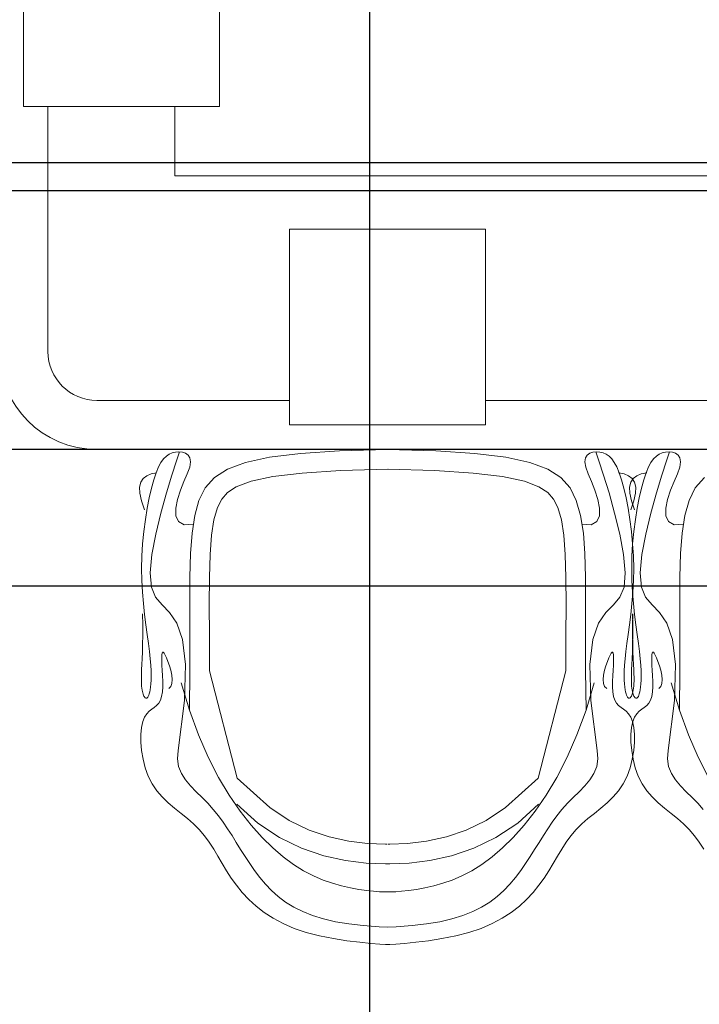
# Model space of a CAD drawing. Units: inches. Extents: x 1454 to 2136, y 626 to 1213.
# Tile 8 of 23: x 1592 to 1620, y 1062 to 1101. Entities that reach past the tile are written whole.
import ezdxf

# ---------------------------------------------------------------- set-up
doc = ezdxf.new("R2010")
doc.units = ezdxf.units.IN
doc.header["$MEASUREMENT"] = 0
for name, color, linetype, lineweight in [('A-ANNO-DIMS', 2, 'Continuous', 18), ('A-FURN-PATT', 252, 'Continuous', 13), ('conference', 41, 'Continuous', 18)]:
    doc.layers.add(name, color=color, linetype=linetype, lineweight=lineweight)
doc.styles.get("Standard").update_dxf_attribs({"font": 'arial.ttf'})
doc.dimstyles.get("Standard").update_dxf_attribs({"dimtxt": 4, "dimasz": 0.18, "dimexe": 0.18, "dimexo": 0.0625, "dimgap": 0.09, "dimtad": 0, "dimtih": 1, "dimtoh": 1, "dimdec": 0, "dimrnd": 6, "dimzin": 0, "dimdsep": 46, "dimlunit": 3, "dimtxsty": 'Standard', "dimcen": 0.09, "dimadec": 0, "dimazin": 0, "dimtfac": 1, "dimtdec": 0, "dimtofl": 0, "dimtmove": 0, "dimatfit": 3, "dimfxl": 1, "dimtolj": 1, "dimtzin": 0, "dimarcsym": 0})

# ---------------------------------------------------------------- blocks, each defined once
blk = doc.blocks.new('ОГ52_на12персон_стол2800х900')
for p, q in [((-1375, -70.7), (-1375, -270.7)), ((-1175, -270.7), (-1175, -70.7)), ((-1375, -270.7), (-1175, -270.7)), ((-1350, -270.7), (-1350, -520.7)), ((-1220.7, -341.4), (-1220.7, -270.7)), ((-1220.7, -341.4), (1220.7, -341.4)), ((-903.4, -395.7), (-1103.4, -395.7)), ((-1103.4, -395.7), (-1103.4, -595.7)), ((-903.4, -595.7), (-903.4, -395.7)), ((-1300, -570.7), (-1103.4, -570.7)), ((-903.4, -570.7), (-603.4, -570.7)), ((-1103.4, -595.7), (-903.4, -595.7)), ((-1300, -620.7), (1300, -620.7)), ((-1216.3, -623.2), (-1219.8, -623.5)), ((-1218.9, -632.3), (-1215.9, -623.2)), ((-1212.8, -623.5), (-1216.3, -623.2)), ((-1092.3, -624.8), (-1052.5, -622.2)), ((-1052.5, -622.2), (-1003.4, -620.7)), ((-954.3, -622.2), (-1003.4, -620.7)), ((-914.4, -624.8), (-954.3, -622.2)), ((-793.9, -623.5), (-790.4, -623.2)), ((-787.8, -632.3), (-790.9, -623.2)), ((-790.4, -623.2), (-786.9, -623.5)), ((-716.3, -623.2), (-719.8, -623.5)), ((-718.9, -632.3), (-715.9, -623.2)), ((-712.8, -623.5), (-716.3, -623.2)), ((-1232, -630.2), (-1234.7, -633.9)), ((-1229.2, -627.4), (-1232, -630.2)), ((-1226.3, -625.5), (-1229.2, -627.4)), ((-1223.2, -624.2), (-1226.3, -625.5)), ((-1223.6, -646.8), (-1218.9, -632.3)), ((-1219.8, -623.5), (-1223.2, -624.2)), ((-1209.6, -624.6), (-1212.8, -623.5)), ((-1207, -626.5), (-1209.6, -624.6)), ((-1205.3, -629.4), (-1207, -626.5)), ((-1204.6, -633.5), (-1205.3, -629.4)), ((-1148.5, -633.9), (-1124, -628.7)), ((-1124, -628.7), (-1092.3, -624.8)), ((-882.8, -628.7), (-914.4, -624.8)), ((-858.3, -633.9), (-882.8, -628.7)), ((-802.1, -633.5), (-801.5, -629.4)), ((-801.5, -629.4), (-799.7, -626.5)), ((-799.7, -626.5), (-797.1, -624.6)), ((-797.1, -624.6), (-793.9, -623.5)), ((-783.1, -646.8), (-787.8, -632.3)), ((-786.9, -623.5), (-783.6, -624.2)), ((-783.6, -624.2), (-780.4, -625.5)), ((-780.4, -625.5), (-777.5, -627.4)), ((-777.5, -627.4), (-774.7, -630.2)), ((-774.7, -630.2), (-772.1, -633.9)), ((-732, -630.2), (-734.7, -633.9)), ((-729.2, -627.4), (-732, -630.2)), ((-726.3, -625.5), (-729.2, -627.4)), ((-723.2, -624.2), (-726.3, -625.5)), ((-723.6, -646.8), (-718.9, -632.3)), ((-719.8, -623.5), (-723.2, -624.2)), ((-709.6, -624.6), (-712.8, -623.5)), ((-707, -626.5), (-709.6, -624.6)), ((-705.3, -629.4), (-707, -626.5)), ((-704.6, -633.5), (-705.3, -629.4)), ((-1237.2, -638.6), (-1239.7, -644.5)), ((-1234.7, -633.9), (-1237.2, -638.6)), ((-1207.8, -645.6), (-1205.4, -638.8)), ((-1205.4, -638.8), (-1204.6, -633.5)), ((-1180.2, -649.4), (-1166.8, -640.7)), ((-1166.8, -640.7), (-1148.5, -633.9)), ((-1090.5, -644.8), (-1051.5, -642.2)), ((-1051.5, -642.2), (-1002.7, -640.7)), ((-955.2, -642.2), (-1004, -640.7)), ((-916.3, -644.8), (-955.2, -642.2)), ((-839.9, -640.7), (-858.3, -633.9)), ((-826.6, -649.4), (-839.9, -640.7)), ((-801.3, -638.8), (-802.1, -633.5)), ((-798.9, -645.6), (-801.3, -638.8)), ((-772.1, -633.9), (-769.5, -638.6)), ((-769.5, -638.6), (-767.1, -644.5)), ((-737.2, -638.6), (-739.7, -644.5)), ((-734.7, -633.9), (-737.2, -638.6)), ((-707.8, -645.6), (-705.4, -638.8)), ((-705.4, -638.8), (-704.6, -633.5)), ((-1255.3, -654.2), (-1252.8, -650.4)), ((-1252.8, -650.4), (-1249.2, -647.6)), ((-1249.2, -647.6), (-1244.6, -645.6)), ((-1244.6, -645.6), (-1239.1, -644.5)), ((-1242.1, -651.7), (-1244.4, -660.3)), ((-1239.7, -644.5), (-1242.1, -651.7)), ((-1229.2, -665.1), (-1223.6, -646.8)), ((-1211.2, -653.4), (-1214.7, -662.3)), ((-1207.8, -645.6), (-1211.2, -653.4)), ((-1189.5, -660), (-1180.2, -649.4)), ((-1157.8, -658.7), (-1142.8, -653.1)), ((-1142.8, -653.1), (-1120.7, -648.4)), ((-1120.7, -648.4), (-1090.5, -644.8)), ((-886.1, -648.4), (-916.3, -644.8)), ((-863.9, -653.1), (-886.1, -648.4)), ((-849, -658.7), (-863.9, -653.1)), ((-817.3, -660), (-826.6, -649.4)), ((-798.9, -645.6), (-795.5, -653.4)), ((-795.5, -653.4), (-792, -662.3)), ((-777.5, -665.1), (-783.1, -646.8)), ((-762.2, -645.6), (-767.7, -644.5)), ((-767.1, -644.5), (-764.7, -651.7)), ((-764.7, -651.7), (-762.3, -660.3)), ((-757.6, -647.6), (-762.2, -645.6)), ((-754, -650.4), (-757.6, -647.6)), ((-755.3, -654.2), (-752.8, -650.4)), ((-751.5, -654.2), (-754, -650.4)), ((-752.8, -650.4), (-749.2, -647.6)), ((-749.2, -647.6), (-744.6, -645.6)), ((-744.6, -645.6), (-739.1, -644.5)), ((-742.1, -651.7), (-744.4, -660.3)), ((-739.7, -644.5), (-742.1, -651.7)), ((-729.2, -665.1), (-723.6, -646.8)), ((-711.2, -653.4), (-714.7, -662.3)), ((-707.8, -645.6), (-711.2, -653.4)), ((-689.5, -660), (-680.2, -649.4)), ((-1256.5, -659.2), (-1255.3, -654.2)), ((-1256.3, -665.5), (-1256.5, -659.2)), ((-1244.4, -660.3), (-1246.6, -670)), ((-1214.7, -662.3), (-1217.7, -671.7)), ((-1195.9, -672.9), (-1189.5, -660)), ((-1166.9, -664.7), (-1157.8, -658.7)), ((-839.8, -664.7), (-849, -658.7)), ((-810.9, -672.9), (-817.3, -660)), ((-792, -662.3), (-789.1, -671.7)), ((-762.3, -660.3), (-760.1, -670)), ((-756.5, -659.2), (-755.3, -654.2)), ((-756.3, -665.5), (-756.5, -659.2)), ((-750.2, -659.2), (-751.5, -654.2)), ((-750.4, -665.5), (-750.2, -659.2)), ((-744.4, -660.3), (-746.6, -670)), ((-714.7, -662.3), (-717.7, -671.7)), ((-695.9, -672.9), (-689.5, -660)), ((-1254.7, -673.2), (-1256.3, -665.5)), ((-1251.4, -682.4), (-1254.7, -673.2)), ((-1246.6, -670), (-1248.7, -680.8)), ((-1235, -685.8), (-1229.2, -665.1)), ((-1217.7, -671.7), (-1219.5, -680.7)), ((-1200.2, -688.1), (-1195.9, -672.9)), ((-1177.1, -680.1), (-1172.7, -671.3)), ((-1172.7, -671.3), (-1166.9, -664.7)), ((-834, -671.3), (-839.8, -664.7)), ((-829.6, -680.1), (-834, -671.3)), ((-806.5, -688.1), (-810.9, -672.9)), ((-789.1, -671.7), (-787.3, -680.7)), ((-771.8, -685.8), (-777.5, -665.1)), ((-760.1, -670), (-758, -680.8)), ((-754.7, -673.2), (-756.3, -665.5)), ((-755.4, -682.4), (-752.1, -673.2)), ((-751.4, -682.4), (-754.7, -673.2)), ((-752.1, -673.2), (-750.4, -665.5)), ((-746.6, -670), (-748.7, -680.8)), ((-735, -685.8), (-729.2, -665.1)), ((-717.7, -671.7), (-719.5, -680.7)), ((-700.2, -688.1), (-695.9, -672.9)), ((-1248.7, -680.8), (-1250.6, -692.3)), ((-1219.5, -680.7), (-1219.4, -688.5)), ((-1180.6, -692.4), (-1177.1, -680.1)), ((-826.1, -692.4), (-829.6, -680.1)), ((-787.3, -680.7), (-787.3, -688.5)), ((-758, -680.8), (-756.2, -692.3)), ((-748.7, -680.8), (-750.6, -692.3)), ((-719.5, -680.7), (-719.4, -688.5)), ((-1250.6, -692.3), (-1252.1, -704.4)), ((-1240.1, -707.3), (-1235, -685.8)), ((-1219.4, -688.5), (-1216.8, -694.3)), ((-1203, -706), (-1200.2, -688.1)), ((-1183.1, -708.3), (-1180.6, -692.4)), ((-823.6, -708.3), (-826.1, -692.4)), ((-803.7, -706), (-806.5, -688.1)), ((-787.3, -688.5), (-789.9, -694.3)), ((-766.6, -707.3), (-771.8, -685.8)), ((-756.2, -692.3), (-754.6, -704.4)), ((-750.6, -692.3), (-752.1, -704.4)), ((-740.1, -707.3), (-735, -685.8)), ((-719.4, -688.5), (-716.8, -694.3)), ((-703, -706), (-700.2, -688.1)), ((-1216.8, -694.3), (-1211.1, -697.5)), ((-1211.1, -697.5), (-1201.6, -697.1)), ((-795.6, -697.5), (-805.1, -697.1)), ((-789.9, -694.3), (-795.6, -697.5)), ((-716.8, -694.3), (-711.1, -697.5)), ((-711.1, -697.5), (-701.6, -697.1)), ((-1252.1, -704.4), (-1253.4, -716.9)), ((-1243.9, -728.1), (-1240.1, -707.3)), ((-1204.6, -726.9), (-1203, -706)), ((-1184.6, -728), (-1183.1, -708.3)), ((-822.1, -728), (-823.6, -708.3)), ((-802.2, -726.9), (-803.7, -706)), ((-762.8, -728.1), (-766.6, -707.3)), ((-754.6, -704.4), (-753.4, -716.9)), ((-752.1, -704.4), (-753.4, -716.9)), ((-743.9, -728.1), (-740.1, -707.3)), ((-704.6, -726.9), (-703, -706)), ((-1253.4, -716.9), (-1254.1, -729.5)), ((-753.4, -716.9), (-754.1, -729.5)), ((-753.4, -716.9), (-752.6, -729.5)), ((-1254.1, -729.5), (-1254.4, -742.1)), ((-1245.6, -746.6), (-1243.9, -728.1)), ((-1205.3, -751.1), (-1204.6, -726.9)), ((-1185.3, -751.4), (-1184.6, -728)), ((-821.5, -751.4), (-822.1, -728)), ((-801.5, -751.1), (-802.2, -726.9)), ((-761.1, -746.6), (-762.8, -728.1)), ((-754.1, -729.5), (-754.4, -742.1)), ((-752.6, -729.5), (-752.3, -742.1)), ((-745.6, -746.6), (-743.9, -728.1)), ((-705.3, -751.1), (-704.6, -726.9)), ((-1254.4, -742.1), (-1254.2, -754.5)), ((-754.4, -742.1), (-754.2, -754.5)), ((-752.3, -742.1), (-752.5, -754.5)), ((-1244.5, -761.4), (-1245.6, -746.6)), ((-1205.4, -778.9), (-1205.3, -751.1)), ((-1185.4, -778.9), (-1185.3, -751.4)), ((-821.4, -778.9), (-821.5, -751.4)), ((-801.4, -778.9), (-801.5, -751.1)), ((-762.2, -761.4), (-761.1, -746.6)), ((-744.5, -761.4), (-745.6, -746.6)), ((-705.4, -778.9), (-705.3, -751.1)), ((-1254.2, -754.5), (-1253.6, -766.5)), ((-1240.2, -771.5), (-1244.5, -761.4)), ((-766.5, -771.5), (-762.2, -761.4)), ((-754.2, -754.5), (-753.6, -766.5)), ((-752.5, -754.5), (-753.1, -766.5)), ((-740.2, -771.5), (-744.5, -761.4)), ((-1253.6, -766.5), (-1252.6, -778.1)), ((-1233.6, -779.2), (-1240.2, -771.5)), ((-773.1, -779.2), (-766.5, -771.5)), ((-753.1, -766.5), (-754.1, -778.1)), ((-753.6, -766.5), (-752.6, -778.1)), ((-733.6, -779.2), (-740.2, -771.5)), ((-1252.6, -778.1), (-1251.4, -789.2)), ((-1226, -787), (-1233.6, -779.2)), ((-1205.3, -810.6), (-1205.4, -778.9)), ((-1185.3, -810.5), (-1185.4, -778.9)), ((-821.5, -810.5), (-821.4, -778.9)), ((-801.5, -810.6), (-801.4, -778.9)), ((-780.7, -787), (-773.1, -779.2)), ((-754.1, -778.1), (-755.4, -789.2)), ((-752.6, -778.1), (-751.4, -789.2)), ((-726, -787), (-733.6, -779.2)), ((-705.3, -810.6), (-705.4, -778.9)), ((-1253.3, -800.2), (-1253.4, -788.5)), ((-1251.4, -789.2), (-1250, -799.7)), ((-1218.6, -798), (-1226, -787)), ((-788.1, -798), (-780.7, -787)), ((-755.4, -789.2), (-756.7, -799.7)), ((-753.5, -800.2), (-753.3, -788.5)), ((-753.3, -800.2), (-753.4, -788.5)), ((-751.4, -789.2), (-750, -799.7)), ((-718.6, -798), (-726, -787)), ((-1253.3, -810.5), (-1253.3, -800.2)), ((-1250, -799.7), (-1248.7, -809.6)), ((-1212.8, -814.7), (-1218.6, -798)), ((-794, -814.7), (-788.1, -798)), ((-756.7, -799.7), (-758, -809.6)), ((-753.4, -810.5), (-753.5, -800.2)), ((-753.3, -810.5), (-753.3, -800.2)), ((-750, -799.7), (-748.7, -809.6)), ((-712.8, -814.7), (-718.6, -798)), ((-1253.4, -819.6), (-1253.3, -810.5)), ((-1248.7, -809.6), (-1247.4, -818.7)), ((-1205.3, -846.4), (-1205.3, -810.6)), ((-1185.3, -846.6), (-1185.3, -810.5)), ((-821.5, -846.6), (-821.5, -810.5)), ((-801.5, -846.4), (-801.5, -810.6)), ((-758, -809.6), (-759.3, -818.7)), ((-753.3, -819.6), (-753.4, -810.5)), ((-753.4, -819.6), (-753.3, -810.5)), ((-748.7, -809.6), (-747.4, -818.7)), ((-705.3, -846.4), (-705.3, -810.6)), ((-1253.7, -827.5), (-1253.4, -819.6)), ((-1247.4, -818.7), (-1246.4, -827)), ((-1209.7, -840.1), (-1212.8, -814.7)), ((-797, -840.1), (-794, -814.7)), ((-759.3, -818.7), (-760.4, -827)), ((-753.7, -827.5), (-753.4, -819.6)), ((-753.1, -827.5), (-753.3, -819.6)), ((-747.4, -818.7), (-746.4, -827)), ((-709.7, -840.1), (-712.8, -814.7)), ((-1254.2, -840.3), (-1253.9, -834.3)), ((-1253.9, -834.3), (-1253.7, -827.5)), ((-1246.4, -827), (-1245.6, -834.4)), ((-1233.8, -830.5), (-1233.9, -833.2)), ((-1233.9, -833.2), (-1233.9, -836.7)), ((-1233.5, -828.6), (-1233.8, -830.5)), ((-1233, -827.7), (-1233.5, -828.6)), ((-1232.3, -827.8), (-1233, -827.7)), ((-1231.4, -828.7), (-1232.3, -827.8)), ((-1230.3, -830.6), (-1231.4, -828.7)), ((-1229, -833.4), (-1230.3, -830.6)), ((-1227.6, -837.1), (-1229, -833.4)), ((-779.2, -837.1), (-777.7, -833.4)), ((-777.7, -833.4), (-776.4, -830.6)), ((-776.4, -830.6), (-775.3, -828.7)), ((-775.3, -828.7), (-774.4, -827.8)), ((-774.4, -827.8), (-773.8, -827.7)), ((-773.8, -827.7), (-773.3, -828.6)), ((-773.3, -828.6), (-772.9, -830.5)), ((-772.9, -830.5), (-772.8, -833.2)), ((-772.8, -833.2), (-772.9, -836.7)), ((-760.4, -827), (-761.2, -834.4)), ((-754.2, -840.3), (-753.9, -834.3)), ((-753.9, -834.3), (-753.7, -827.5)), ((-752.8, -834.3), (-753.1, -827.5)), ((-752.5, -840.3), (-752.8, -834.3)), ((-746.4, -827), (-745.6, -834.4)), ((-733.8, -830.5), (-733.9, -833.2)), ((-733.9, -833.2), (-733.9, -836.7)), ((-733.5, -828.6), (-733.8, -830.5)), ((-733, -827.7), (-733.5, -828.6)), ((-732.3, -827.8), (-733, -827.7)), ((-731.4, -828.7), (-732.3, -827.8)), ((-730.3, -830.6), (-731.4, -828.7)), ((-729, -833.4), (-730.3, -830.6)), ((-727.6, -837.1), (-729, -833.4)), ((-1254.5, -845.4), (-1254.2, -840.3)), ((-1245.6, -834.4), (-1245.1, -841)), ((-1245.1, -841), (-1244.8, -846.8)), ((-1233.9, -836.7), (-1233.7, -841.2)), ((-1233.7, -841.2), (-1233.4, -846.2)), ((-1226.1, -841.5), (-1227.6, -837.1)), ((-1224.7, -846.2), (-1226.1, -841.5)), ((-1210.8, -876.9), (-1209.7, -840.1)), ((-796, -876.9), (-797, -840.1)), ((-782, -846.2), (-780.7, -841.5)), ((-780.7, -841.5), (-779.2, -837.1)), ((-773.1, -841.2), (-773.4, -846.2)), ((-772.9, -836.7), (-773.1, -841.2)), ((-761.7, -841), (-762, -846.8)), ((-761.2, -834.4), (-761.7, -841)), ((-754.5, -845.4), (-754.2, -840.3)), ((-752.3, -845.4), (-752.5, -840.3)), ((-745.6, -834.4), (-745.1, -841)), ((-745.1, -841), (-744.8, -846.8)), ((-733.9, -836.7), (-733.7, -841.2)), ((-733.7, -841.2), (-733.4, -846.2)), ((-726.1, -841.5), (-727.6, -837.1)), ((-724.7, -846.2), (-726.1, -841.5)), ((-710.8, -876.9), (-709.7, -840.1)), ((-1254.7, -853.7), (-1254.6, -849.8)), ((-1254.7, -857), (-1254.7, -853.7)), ((-1254.6, -849.8), (-1254.5, -845.4)), ((-1244.8, -846.8), (-1244.7, -851.9)), ((-1244.7, -851.9), (-1244.8, -856.3)), ((-1233.4, -846.2), (-1233.1, -851.7)), ((-1233.1, -851.7), (-1232.9, -857.3)), ((-1223.7, -851), (-1224.7, -846.2)), ((-1223.3, -855.5), (-1223.7, -851)), ((-1205.7, -886.8), (-1205.3, -846.4)), ((-1157, -956.4), (-1185.3, -846.6)), ((-849.8, -956.4), (-821.5, -846.6)), ((-801, -886.8), (-801.5, -846.4)), ((-783.5, -855.5), (-783, -851)), ((-783, -851), (-782, -846.2)), ((-773.6, -851.7), (-773.8, -857.3)), ((-773.4, -846.2), (-773.6, -851.7)), ((-762, -846.8), (-762, -851.9)), ((-762, -851.9), (-761.9, -856.3)), ((-754.7, -853.7), (-754.6, -849.8)), ((-754.7, -857), (-754.7, -853.7)), ((-754.6, -849.8), (-754.5, -845.4)), ((-752.1, -849.8), (-752.3, -845.4)), ((-752, -853.7), (-752.1, -849.8)), ((-752, -857), (-752, -853.7)), ((-744.8, -846.8), (-744.7, -851.9)), ((-744.7, -851.9), (-744.8, -856.3)), ((-733.4, -846.2), (-733.1, -851.7)), ((-733.1, -851.7), (-732.9, -857.3)), ((-723.7, -851), (-724.7, -846.2)), ((-723.3, -855.5), (-723.7, -851)), ((-705.7, -886.8), (-705.3, -846.4)), ((-1254.6, -859.9), (-1254.7, -857)), ((-1254.5, -862.4), (-1254.6, -859.9)), ((-1254.2, -864.5), (-1254.5, -862.4)), ((-1254, -866.3), (-1254.2, -864.5)), ((-1245.3, -863.3), (-1245.7, -866)), ((-1245, -860.1), (-1245.3, -863.3)), ((-1244.8, -856.3), (-1245, -860.1)), ((-1232.9, -862.9), (-1233.3, -868.2)), ((-1232.9, -857.3), (-1232.9, -862.9)), ((-1226.8, -864.8), (-1224.6, -862.7)), ((-1224.6, -862.7), (-1223.5, -859.6)), ((-1223.5, -859.6), (-1223.3, -855.5)), ((-1214, -859), (-1205.7, -886.8)), ((-792.7, -859), (-801, -886.8)), ((-783.2, -859.6), (-783.5, -855.5)), ((-782.1, -862.7), (-783.2, -859.6)), ((-779.9, -864.8), (-782.1, -862.7)), ((-773.8, -857.3), (-773.8, -862.9)), ((-773.8, -862.9), (-773.5, -868.2)), ((-761.9, -856.3), (-761.7, -860.1)), ((-761.7, -860.1), (-761.4, -863.3)), ((-761.4, -863.3), (-761, -866)), ((-754.6, -859.9), (-754.7, -857)), ((-754.5, -862.4), (-754.6, -859.9)), ((-754.2, -864.5), (-754.5, -862.4)), ((-754, -866.3), (-754.2, -864.5)), ((-752.8, -866.3), (-752.5, -864.5)), ((-752.5, -864.5), (-752.3, -862.4)), ((-752.3, -862.4), (-752.1, -859.9)), ((-752.1, -859.9), (-752, -857)), ((-745.3, -863.3), (-745.7, -866)), ((-745, -860.1), (-745.3, -863.3)), ((-744.8, -856.3), (-745, -860.1)), ((-732.9, -862.9), (-733.3, -868.2)), ((-732.9, -857.3), (-732.9, -862.9)), ((-726.8, -864.8), (-724.6, -862.7)), ((-724.6, -862.7), (-723.5, -859.6)), ((-723.5, -859.6), (-723.3, -855.5)), ((-714, -859), (-705.7, -886.8)), ((-1253.6, -867.9), (-1254, -866.3)), ((-1253.3, -869.2), (-1253.6, -867.9)), ((-1252.9, -870.5), (-1253.3, -869.2)), ((-1252.5, -871.6), (-1252.9, -870.5)), ((-1252.1, -872.5), (-1252.5, -871.6)), ((-1251.6, -873.3), (-1252.1, -872.5)), ((-1251.2, -873.9), (-1251.6, -873.3)), ((-1250.7, -874.3), (-1251.2, -873.9)), ((-1250.2, -874.6), (-1250.7, -874.3)), ((-1248.7, -874.3), (-1249.2, -874.6)), ((-1248.1, -873.7), (-1248.7, -874.3)), ((-1247.6, -872.9), (-1248.1, -873.7)), ((-1247.1, -871.7), (-1247.6, -872.9)), ((-1246.6, -870.2), (-1247.1, -871.7)), ((-1246.2, -868.3), (-1246.6, -870.2)), ((-1245.7, -866), (-1246.2, -868.3)), ((-1234, -872.9), (-1235.2, -876.8)), ((-1233.3, -868.2), (-1234, -872.9)), ((-773.5, -868.2), (-772.8, -872.9)), ((-772.8, -872.9), (-771.6, -876.8)), ((-761, -866), (-760.6, -868.3)), ((-760.6, -868.3), (-760.1, -870.2)), ((-760.1, -870.2), (-759.6, -871.7)), ((-759.6, -871.7), (-759.1, -872.9)), ((-759.1, -872.9), (-758.6, -873.7)), ((-758.6, -873.7), (-758.1, -874.3)), ((-758.1, -874.3), (-757.6, -874.6)), ((-756.5, -874.6), (-756, -874.3)), ((-756, -874.3), (-755.6, -873.9)), ((-755.6, -873.9), (-755.1, -873.3)), ((-755.1, -873.3), (-754.7, -872.5)), ((-754.7, -872.5), (-754.2, -871.6)), ((-754.2, -871.6), (-753.8, -870.5)), ((-753.6, -867.9), (-754, -866.3)), ((-753.8, -870.5), (-753.5, -869.2)), ((-753.3, -869.2), (-753.6, -867.9)), ((-753.5, -869.2), (-753.1, -867.9)), ((-752.9, -870.5), (-753.3, -869.2)), ((-753.1, -867.9), (-752.8, -866.3)), ((-752.5, -871.6), (-752.9, -870.5)), ((-752.1, -872.5), (-752.5, -871.6)), ((-751.6, -873.3), (-752.1, -872.5)), ((-751.2, -873.9), (-751.6, -873.3)), ((-750.7, -874.3), (-751.2, -873.9)), ((-750.2, -874.6), (-750.7, -874.3)), ((-748.7, -874.3), (-749.2, -874.6)), ((-748.1, -873.7), (-748.7, -874.3)), ((-747.6, -872.9), (-748.1, -873.7)), ((-747.1, -871.7), (-747.6, -872.9)), ((-746.6, -870.2), (-747.1, -871.7)), ((-746.2, -868.3), (-746.6, -870.2)), ((-745.7, -866), (-746.2, -868.3)), ((-734, -872.9), (-735.2, -876.8)), ((-733.3, -868.2), (-734, -872.9)), ((-1249.7, -874.7), (-1250.2, -874.6)), ((-1249.2, -874.6), (-1249.7, -874.7)), ((-1241.5, -884.1), (-1244.1, -886)), ((-1239.1, -882.2), (-1241.5, -884.1)), ((-1236.9, -879.9), (-1239.1, -882.2)), ((-1235.2, -876.8), (-1236.9, -879.9)), ((-1217.1, -927.9), (-1210.8, -876.9)), ((-789.6, -927.9), (-796, -876.9)), ((-771.6, -876.8), (-769.8, -879.9)), ((-769.8, -879.9), (-767.7, -882.2)), ((-767.7, -882.2), (-765.2, -884.1)), ((-765.2, -884.1), (-762.6, -886)), ((-757.6, -874.6), (-757, -874.7)), ((-757, -874.7), (-756.5, -874.6)), ((-749.7, -874.7), (-750.2, -874.6)), ((-749.2, -874.6), (-749.7, -874.7)), ((-741.5, -884.1), (-744.1, -886)), ((-739.1, -882.2), (-741.5, -884.1)), ((-736.9, -879.9), (-739.1, -882.2)), ((-735.2, -876.8), (-736.9, -879.9)), ((-717.1, -927.9), (-710.8, -876.9)), ((-1251.4, -894), (-1253.2, -898.6)), ((-1249.2, -890.6), (-1251.4, -894)), ((-1246.7, -888), (-1249.2, -890.6)), ((-1244.1, -886), (-1246.7, -888)), ((-1205.7, -886.8), (-1196.5, -912.1)), ((-801, -886.8), (-810.2, -912.1)), ((-762.6, -886), (-760, -888)), ((-760, -888), (-757.5, -890.6)), ((-757.5, -890.6), (-755.3, -894)), ((-755.3, -894), (-753.5, -898.6)), ((-751.4, -894), (-753.2, -898.6)), ((-749.2, -890.6), (-751.4, -894)), ((-746.7, -888), (-749.2, -890.6)), ((-744.1, -886), (-746.7, -888)), ((-705.7, -886.8), (-696.5, -912.1)), ((-1254.5, -904.5), (-1255.1, -911.6)), ((-1253.2, -898.6), (-1254.5, -904.5)), ((-754.5, -904.5), (-755.1, -911.6)), ((-753.2, -898.6), (-754.5, -904.5)), ((-753.5, -898.6), (-752.3, -904.5)), ((-752.3, -904.5), (-751.6, -911.6)), ((-1255.1, -911.6), (-1255.1, -919.5)), ((-1196.5, -912.1), (-1186.6, -934.9)), ((-810.2, -912.1), (-820.1, -934.9)), ((-755.1, -911.6), (-755.1, -919.5)), ((-751.6, -911.6), (-751.6, -919.5)), ((-696.5, -912.1), (-686.6, -934.9)), ((-1255.1, -919.5), (-1254.4, -928)), ((-755.1, -919.5), (-754.4, -928)), ((-751.6, -919.5), (-752.3, -928)), ((-1254.4, -928), (-1253, -936.8)), ((-1217.1, -927.9), (-1217.9, -936.5)), ((-789.6, -927.9), (-788.8, -936.5)), ((-754.4, -928), (-753, -936.8)), ((-752.3, -928), (-753.8, -936.8)), ((-717.1, -927.9), (-717.9, -936.5)), ((-1253, -936.8), (-1250.7, -945.6)), ((-1217.9, -936.5), (-1216.7, -944.3)), ((-1216.7, -944.3), (-1213.8, -951.4)), ((-1186.6, -934.9), (-1176.1, -955.5)), ((-820.1, -934.9), (-830.7, -955.5)), ((-790, -944.3), (-792.9, -951.4)), ((-788.8, -936.5), (-790, -944.3)), ((-753.8, -936.8), (-756, -945.6)), ((-753, -936.8), (-750.7, -945.6)), ((-717.9, -936.5), (-716.7, -944.3)), ((-716.7, -944.3), (-713.8, -951.4)), ((-686.6, -934.9), (-676.1, -955.5)), ((-1250.7, -945.6), (-1247.7, -954.1)), ((-1247.7, -954.1), (-1243.7, -962)), ((-1213.8, -951.4), (-1209.6, -958)), ((-792.9, -951.4), (-797.1, -958)), ((-759.1, -954.1), (-763, -962)), ((-756, -945.6), (-759.1, -954.1)), ((-750.7, -945.6), (-747.7, -954.1)), ((-747.7, -954.1), (-743.7, -962)), ((-713.8, -951.4), (-709.6, -958)), ((-1243.7, -962), (-1238.9, -969.1)), ((-1209.6, -958), (-1204.5, -964.1)), ((-1204.5, -964.1), (-1198.7, -970.1)), ((-1176.1, -955.5), (-1165.2, -973.8)), ((-1157, -956.4), (-1123.7, -986.3)), ((-849.8, -956.4), (-883, -986.3)), ((-830.7, -955.5), (-841.6, -973.8)), ((-802.3, -964.1), (-808, -970.1)), ((-797.1, -958), (-802.3, -964.1)), ((-763, -962), (-767.8, -969.1)), ((-743.7, -962), (-738.9, -969.1)), ((-709.6, -958), (-704.5, -964.1)), ((-704.5, -964.1), (-698.7, -970.1)), ((-1238.9, -969.1), (-1233.4, -975.5)), ((-1198.7, -970.1), (-1192.7, -976)), ((-1165.2, -973.8), (-1154, -990)), ((-841.6, -973.8), (-852.8, -990)), ((-808, -970.1), (-814.1, -976)), ((-767.8, -969.1), (-773.4, -975.5)), ((-738.9, -969.1), (-733.4, -975.5)), ((-698.7, -970.1), (-692.7, -976)), ((-1233.4, -975.5), (-1227.3, -981.4)), ((-1227.3, -981.4), (-1220.8, -986.9)), ((-1192.7, -976), (-1186.8, -982)), ((-1186.8, -982), (-1181.3, -988.2)), ((-1157.3, -983), (-1136, -1002.1)), ((-849.4, -983), (-870.7, -1002.1)), ((-820, -982), (-825.5, -988.2)), ((-814.1, -976), (-820, -982)), ((-779.5, -981.4), (-785.9, -986.9)), ((-773.4, -975.5), (-779.5, -981.4)), ((-733.4, -975.5), (-727.3, -981.4)), ((-727.3, -981.4), (-720.8, -986.9)), ((-692.7, -976), (-686.8, -982)), ((-686.8, -982), (-681.3, -988.2)), ((-1220.8, -986.9), (-1214.2, -992.3)), ((-1214.2, -992.3), (-1207.7, -997.6)), ((-1181.3, -988.2), (-1176.1, -994.6)), ((-1176.1, -994.6), (-1171.3, -1001.3)), ((-1154, -990), (-1142.7, -1004.3)), ((-1123.7, -986.3), (-1103.8, -999.5)), ((-883, -986.3), (-902.9, -999.5)), ((-852.8, -990), (-864, -1004.3)), ((-830.6, -994.6), (-835.5, -1001.3)), ((-825.5, -988.2), (-830.6, -994.6)), ((-792.5, -992.3), (-799, -997.6)), ((-785.9, -986.9), (-792.5, -992.3)), ((-720.8, -986.9), (-714.2, -992.3)), ((-714.2, -992.3), (-707.7, -997.6)), ((-1207.7, -997.6), (-1201.4, -1003)), ((-1201.4, -1003), (-1195.6, -1008.8)), ((-1171.3, -1001.3), (-1166.7, -1008.1)), ((-1142.7, -1004.3), (-1131.5, -1016.8)), ((-1136, -1002.1), (-1113.8, -1016.9)), ((-1103.8, -999.5), (-1083.6, -1009.3)), ((-902.9, -999.5), (-923.2, -1009.3)), ((-870.7, -1002.1), (-893, -1016.9)), ((-864, -1004.3), (-875.2, -1016.8)), ((-835.5, -1001.3), (-840.1, -1008.1)), ((-805.3, -1003), (-811.2, -1008.8)), ((-799, -997.6), (-805.3, -1003)), ((-707.7, -997.6), (-701.4, -1003)), ((-701.4, -1003), (-695.6, -1008.8)), ((-1195.6, -1008.8), (-1190.3, -1015.1)), ((-1190.3, -1015.1), (-1185.4, -1021.7)), ((-1166.7, -1008.1), (-1162.2, -1015)), ((-1162.2, -1015), (-1157.8, -1022.1)), ((-1083.6, -1009.3), (-1063.2, -1016.2)), ((-923.2, -1009.3), (-943.5, -1016.2)), ((-844.5, -1015), (-848.9, -1022.1)), ((-840.1, -1008.1), (-844.5, -1015)), ((-816.5, -1015.1), (-821.3, -1021.7)), ((-811.2, -1008.8), (-816.5, -1015.1)), ((-695.6, -1008.8), (-690.3, -1015.1)), ((-690.3, -1015.1), (-685.4, -1021.7)), ((-1185.4, -1021.7), (-1180.9, -1028.7)), ((-1157.8, -1022.1), (-1153.4, -1029.2)), ((-1131.5, -1016.8), (-1120.6, -1027.5)), ((-1113.8, -1016.9), (-1091.2, -1027.9)), ((-1063.2, -1016.2), (-1043.1, -1020.6)), ((-1043.1, -1020.6), (-1023.8, -1023)), ((-1023.8, -1023), (-1005.5, -1023.8)), ((-1005.5, -1023.8), (-1003.8, -1023.8)), ((-1001.3, -1023.8), (-1003, -1023.8)), ((-983, -1023), (-1001.3, -1023.8)), ((-963.6, -1020.6), (-983, -1023)), ((-943.5, -1016.2), (-963.6, -1020.6)), ((-893, -1016.9), (-915.6, -1027.9)), ((-875.2, -1016.8), (-886.2, -1027.5)), ((-848.9, -1022.1), (-853.4, -1029.2)), ((-821.3, -1021.7), (-825.8, -1028.7)), ((-685.4, -1021.7), (-680.9, -1028.7)), ((-1180.9, -1028.7), (-1176.6, -1035.9)), ((-1153.4, -1029.2), (-1148.8, -1036.4)), ((-1120.6, -1027.5), (-1109.9, -1036.7)), ((-1091.2, -1027.9), (-1068.6, -1035.5)), ((-915.6, -1027.9), (-938.1, -1035.5)), ((-886.2, -1027.5), (-896.9, -1036.7)), ((-853.4, -1029.2), (-857.9, -1036.4)), ((-825.8, -1028.7), (-830.2, -1035.9)), ((-1176.6, -1035.9), (-1172.2, -1043.3)), ((-1172.2, -1043.3), (-1167.7, -1050.8)), ((-1148.8, -1036.4), (-1144.1, -1043.6)), ((-1144.1, -1043.6), (-1139.2, -1050.7)), ((-1109.9, -1036.7), (-1099.4, -1044.4)), ((-1099.4, -1044.4), (-1089.1, -1050.8)), ((-1068.6, -1035.5), (-1046.5, -1040.4)), ((-1046.5, -1040.4), (-1025.4, -1043)), ((-1025.4, -1043), (-1005.7, -1043.8)), ((-1005.7, -1043.8), (-1003.4, -1043.8)), ((-1001, -1043.8), (-1003.4, -1043.8)), ((-981.3, -1043), (-1001, -1043.8)), ((-960.2, -1040.4), (-981.3, -1043)), ((-938.1, -1035.5), (-960.2, -1040.4)), ((-907.4, -1044.4), (-917.6, -1050.8)), ((-896.9, -1036.7), (-907.4, -1044.4)), ((-862.6, -1043.6), (-867.6, -1050.7)), ((-857.9, -1036.4), (-862.6, -1043.6)), ((-834.5, -1043.3), (-839, -1050.8)), ((-830.2, -1035.9), (-834.5, -1043.3)), ((-1167.7, -1050.8), (-1162.9, -1058.3)), ((-1139.2, -1050.7), (-1133.9, -1057.7)), ((-1089.1, -1050.8), (-1079.1, -1056)), ((-917.6, -1050.8), (-927.6, -1056)), ((-867.6, -1050.7), (-872.9, -1057.7)), ((-839, -1050.8), (-843.8, -1058.3)), ((-1162.9, -1058.3), (-1157.6, -1065.7)), ((-1133.9, -1057.7), (-1128.1, -1064.5)), ((-1128.1, -1064.5), (-1121.9, -1071)), ((-1079.1, -1056), (-1069.3, -1060.3)), ((-1069.3, -1060.3), (-1059.7, -1063.6)), ((-1059.7, -1063.6), (-1050.4, -1066.3)), ((-947, -1063.6), (-956.3, -1066.3)), ((-937.4, -1060.3), (-947, -1063.6)), ((-927.6, -1056), (-937.4, -1060.3)), ((-878.6, -1064.5), (-884.9, -1071)), ((-872.9, -1057.7), (-878.6, -1064.5)), ((-843.8, -1058.3), (-849.1, -1065.7)), ((-1157.6, -1065.7), (-1151.7, -1073)), ((-1151.7, -1073), (-1145.1, -1080.1)), ((-1121.9, -1071), (-1115, -1077.1)), ((-1050.4, -1066.3), (-1041.3, -1068.3)), ((-1041.3, -1068.3), (-1032.7, -1069.9)), ((-1032.7, -1069.9), (-1024.7, -1071)), ((-1024.7, -1071), (-1017.7, -1071.7)), ((-1017.7, -1071.7), (-1011.8, -1072.2)), ((-1011.8, -1072.2), (-1007.3, -1072.4)), ((-1007.3, -1072.4), (-1004.4, -1072.5)), ((-1004.4, -1072.5), (-1003.4, -1072.5)), ((-1002.3, -1072.5), (-1003.4, -1072.5)), ((-999.4, -1072.4), (-1002.3, -1072.5)), ((-994.9, -1072.2), (-999.4, -1072.4)), ((-989.1, -1071.7), (-994.9, -1072.2)), ((-982, -1071), (-989.1, -1071.7)), ((-974.1, -1069.9), (-982, -1071)), ((-965.4, -1068.3), (-974.1, -1069.9)), ((-956.3, -1066.3), (-965.4, -1068.3)), ((-884.9, -1071), (-891.7, -1077.1)), ((-855, -1073), (-861.6, -1080.1)), ((-849.1, -1065.7), (-855, -1073)), ((-1145.1, -1080.1), (-1137.7, -1086.9)), ((-1115, -1077.1), (-1107.5, -1082.8)), ((-1107.5, -1082.8), (-1099.2, -1088)), ((-899.2, -1082.8), (-907.5, -1088)), ((-891.7, -1077.1), (-899.2, -1082.8)), ((-861.6, -1080.1), (-869, -1086.9)), ((-1137.7, -1086.9), (-1129.5, -1093.3)), ((-1129.5, -1093.3), (-1120.3, -1099.3)), ((-1099.2, -1088), (-1090.1, -1092.6)), ((-1090.1, -1092.6), (-1080, -1096.6)), ((-916.6, -1092.6), (-926.7, -1096.6)), ((-907.5, -1088), (-916.6, -1092.6)), ((-877.3, -1093.3), (-886.5, -1099.3)), ((-869, -1086.9), (-877.3, -1093.3)), ((-1120.3, -1099.3), (-1110.1, -1104.8)), ((-1110.1, -1104.8), (-1098.8, -1109.7)), ((-1080, -1096.6), (-1068.9, -1100)), ((-1068.9, -1100), (-1056.7, -1102.9)), ((-1056.7, -1102.9), (-1043.1, -1105.2)), ((-1043.1, -1105.2), (-1028.3, -1106.9)), ((-963.6, -1105.2), (-978.4, -1106.9)), ((-950.1, -1102.9), (-963.6, -1105.2)), ((-937.8, -1100), (-950.1, -1102.9)), ((-926.7, -1096.6), (-937.8, -1100)), ((-896.6, -1104.8), (-907.9, -1109.7)), ((-886.5, -1099.3), (-896.6, -1104.8)), ((-1098.8, -1109.7), (-1086.4, -1113.9)), ((-1086.4, -1113.9), (-1072.8, -1117.3)), ((-1028.3, -1106.9), (-1012, -1108.1)), ((-1012, -1108.1), (-1003.4, -1108.4)), ((-994.8, -1108.1), (-1003.4, -1108.4)), ((-978.4, -1106.9), (-994.8, -1108.1)), ((-920.4, -1113.9), (-933.9, -1117.3)), ((-907.9, -1109.7), (-920.4, -1113.9)), ((-1072.8, -1117.3), (-1058.8, -1120.1)), ((-1058.8, -1120.1), (-1044.9, -1122.3)), ((-1044.9, -1122.3), (-1031.9, -1123.9)), ((-1031.9, -1123.9), (-1020.6, -1125.1)), ((-1020.6, -1125.1), (-1011.5, -1125.8)), ((-1011.5, -1125.8), (-1005.6, -1126.2)), ((-995.2, -1125.8), (-1001.2, -1126.2)), ((-986.2, -1125.1), (-995.2, -1125.8)), ((-974.8, -1123.9), (-986.2, -1125.1)), ((-961.8, -1122.3), (-974.8, -1123.9)), ((-948, -1120.1), (-961.8, -1122.3)), ((-933.9, -1117.3), (-948, -1120.1)), ((-1005.6, -1126.2), (-1003.4, -1126.3)), ((-1001.2, -1126.2), (-1003.4, -1126.3))]:
    blk.add_line(p, q)
for radius in [100, 50]:
    blk.add_arc((-1300, -520.7), radius, 180, 270)
blk = doc.blocks.new('*D33')
at = {"layer": 'A-ANNO-DIMS', "color": 0, "lineweight": -2, "transparency": 16777216}
for p, q in [((2032.494, 1126.282), (1462.374, 1126.282)), ((1462.554, 1126.102), (1462.554, 1056.381)), ((1462.554, 982.462), (1462.554, 1052.184)), ((2032.494, 982.282), (1462.374, 982.282))]:
    blk.add_line(p, q, dxfattribs=at)
at = {"layer": 'A-ANNO-DIMS', "color": 0, "transparency": 16777216}
for points in [[(1462.524, 1126.102), (1462.584, 1126.102), (1462.554, 1126.282)], [(1462.524, 982.462), (1462.584, 982.462), (1462.554, 982.282)]]:
    blk.add_solid(points, dxfattribs=at)
at = {"layer": 'Defpoints', "color": 0, "transparency": 16777216}
for p in [(1462.554, 1126.282), (2032.556, 1126.282), (2032.556, 982.282)]:
    blk.add_point(p, dxfattribs=at)
at = {"layer": 'A-ANNO-DIMS', "color": 0, "transparency": 16777216, "insert": (1462.554, 1054.282), "char_height": 4, "attachment_point": 5}
blk.add_mtext('\\A1;144', dxfattribs=at)
blk = doc.blocks.new('*D40')
at = {"layer": 'A-ANNO-DIMS', "color": 0, "lineweight": -2, "transparency": 16777216}
for p, q in [((1501.556, 877.345), (1501.556, 1210.464)), ((1501.736, 1210.284), (1569.244, 1210.284)), ((1645.376, 1210.284), (1577.869, 1210.284)), ((1645.556, 877.345), (1645.556, 1210.464))]:
    blk.add_line(p, q, dxfattribs=at)
at = {"layer": 'A-ANNO-DIMS', "color": 0, "transparency": 16777216}
for points in [[(1501.736, 1210.314), (1501.736, 1210.254), (1501.556, 1210.284)], [(1645.376, 1210.314), (1645.376, 1210.254), (1645.556, 1210.284)]]:
    blk.add_solid(points, dxfattribs=at)
at = {"layer": 'Defpoints', "color": 0, "transparency": 16777216}
for p in [(1645.556, 1210.284), (1501.556, 877.282), (1645.556, 877.282)]:
    blk.add_point(p, dxfattribs=at)
at = {"layer": 'A-ANNO-DIMS', "color": 0, "transparency": 16777216, "insert": (1573.556, 1210.284), "char_height": 4, "attachment_point": 5}
blk.add_mtext('\\A1;144', dxfattribs=at)
blk = doc.blocks.new('*D54')
at = {"layer": 'A-ANNO-DIMS', "color": 0, "lineweight": -2, "transparency": 16777216}
for p, q in [((1879.494, 1126.282), (1462.374, 1126.282)), ((1462.554, 1126.102), (1462.554, 1078.915)), ((1462.554, 1027.462), (1462.554, 1074.65)), ((1879.494, 1027.282), (1462.374, 1027.282))]:
    blk.add_line(p, q, dxfattribs=at)
at = {"layer": 'A-ANNO-DIMS', "color": 0, "transparency": 16777216}
for points in [[(1462.524, 1126.102), (1462.584, 1126.102), (1462.554, 1126.282)], [(1462.524, 1027.462), (1462.584, 1027.462), (1462.554, 1027.282)]]:
    blk.add_solid(points, dxfattribs=at)
at = {"layer": 'Defpoints', "color": 0, "transparency": 16777216}
for p in [(1879.556, 1126.282), (1462.554, 1027.282), (1879.556, 1027.282)]:
    blk.add_point(p, dxfattribs=at)
at = {"layer": 'A-ANNO-DIMS', "color": 0, "transparency": 16777216, "insert": (1462.554, 1076.782), "char_height": 4, "attachment_point": 5}
blk.add_mtext('\\A1;99', dxfattribs=at)
blk = doc.blocks.new('*D67')
at = {"layer": 'A-ANNO-DIMS', "color": 0, "lineweight": -2, "transparency": 16777216}
for p, q in [((1606.484, 1018.345), (1606.484, 1210.464)), ((1606.664, 1210.284), (1610.595, 1210.284)), ((1624.703, 1210.284), (1620.773, 1210.284)), ((1624.883, 1018.329), (1624.883, 1210.464))]:
    blk.add_line(p, q, dxfattribs=at)
at = {"layer": 'A-ANNO-DIMS', "color": 0, "transparency": 16777216}
for points in [[(1606.664, 1210.314), (1606.664, 1210.254), (1606.484, 1210.284)], [(1624.703, 1210.314), (1624.703, 1210.254), (1624.883, 1210.284)]]:
    blk.add_solid(points, dxfattribs=at)
at = {"layer": 'Defpoints', "color": 0, "transparency": 16777216}
for p in [(1624.883, 1210.284), (1606.484, 1018.282), (1624.883, 1018.267)]:
    blk.add_point(p, dxfattribs=at)
at = {"layer": 'A-ANNO-DIMS', "color": 0, "transparency": 16777216, "insert": (1615.684, 1210.284), "char_height": 4, "attachment_point": 5}
blk.add_mtext('\\A1;18.4', dxfattribs=at)
blk = doc.blocks.new('*D70')
at = {"layer": 'A-ANNO-DIMS', "color": 0, "lineweight": -2, "transparency": 16777216}
for p, q in [((1811.166, 1094.525), (1462.374, 1094.525)), ((1462.554, 1094.345), (1462.554, 1088.71)), ((1462.554, 1078.811), (1462.554, 1084.445)), ((1811.166, 1078.631), (1462.374, 1078.631))]:
    blk.add_line(p, q, dxfattribs=at)
at = {"layer": 'A-ANNO-DIMS', "color": 0, "transparency": 16777216}
for points in [[(1462.524, 1094.345), (1462.584, 1094.345), (1462.554, 1094.525)], [(1462.524, 1078.811), (1462.584, 1078.811), (1462.554, 1078.631)]]:
    blk.add_solid(points, dxfattribs=at)
at = {"layer": 'Defpoints', "color": 0, "transparency": 16777216}
for p in [(1462.554, 1094.525), (1811.229, 1094.525), (1811.229, 1078.631)]:
    blk.add_point(p, dxfattribs=at)
at = {"layer": 'A-ANNO-DIMS', "color": 0, "transparency": 16777216, "insert": (1462.554, 1086.578), "char_height": 4, "attachment_point": 5}
blk.add_mtext('\\A1;15.894', dxfattribs=at)
blk = doc.blocks.new('*D73')
at = {"layer": 'A-ANNO-DIMS', "color": 0, "lineweight": -2, "transparency": 16777216}
for p, q in [((1985.096, 1126.439), (1462.374, 1126.439)), ((1462.554, 1126.259), (1462.554, 1113.178)), ((1462.554, 1095.83), (1462.554, 1108.911)), ((1966.644, 1095.65), (1462.374, 1095.65))]:
    blk.add_line(p, q, dxfattribs=at)
at = {"layer": 'A-ANNO-DIMS', "color": 0, "transparency": 16777216}
for points in [[(1462.524, 1126.259), (1462.584, 1126.259), (1462.554, 1126.439)], [(1462.524, 1095.83), (1462.584, 1095.83), (1462.554, 1095.65)]]:
    blk.add_solid(points, dxfattribs=at)
at = {"layer": 'Defpoints', "color": 0, "transparency": 16777216}
for p in [(1985.158, 1126.439), (1462.554, 1095.65), (1966.707, 1095.65)]:
    blk.add_point(p, dxfattribs=at)
at = {"layer": 'A-ANNO-DIMS', "color": 0, "transparency": 16777216, "insert": (1462.554, 1111.044), "char_height": 4, "attachment_point": 5}
blk.add_mtext('\\A1;30.79', dxfattribs=at)
blk = doc.blocks.new('*D76')
at = {"layer": 'A-ANNO-DIMS', "color": 0, "lineweight": -2, "transparency": 16777216}
for p, q in [((1962.644, 1095.65), (1462.374, 1095.65)), ((1462.554, 1095.47), (1462.554, 1073.782)), ((1462.554, 1047.83), (1462.554, 1069.517)), ((1914.644, 1047.65), (1462.374, 1047.65))]:
    blk.add_line(p, q, dxfattribs=at)
at = {"layer": 'A-ANNO-DIMS', "color": 0, "transparency": 16777216}
for points in [[(1462.524, 1095.47), (1462.584, 1095.47), (1462.554, 1095.65)], [(1462.524, 1047.83), (1462.584, 1047.83), (1462.554, 1047.65)]]:
    blk.add_solid(points, dxfattribs=at)
at = {"layer": 'Defpoints', "color": 0, "transparency": 16777216}
for p in [(1962.707, 1095.65), (1462.554, 1047.65), (1914.707, 1047.65)]:
    blk.add_point(p, dxfattribs=at)
at = {"layer": 'A-ANNO-DIMS', "color": 0, "transparency": 16777216, "insert": (1462.554, 1071.65), "char_height": 4, "attachment_point": 5}
blk.add_mtext('\\A1;48', dxfattribs=at)
blk = doc.blocks.new('*D82')
at = {"layer": 'A-ANNO-DIMS', "color": 0, "lineweight": -2, "transparency": 16777216}
for p, q in [((1697.818, 1084.129), (1462.374, 1084.129)), ((1462.554, 1083.949), (1462.554, 1057.83)), ((1462.554, 1027.447), (1462.554, 1053.565)), ((1704.245, 1027.267), (1462.374, 1027.267))]:
    blk.add_line(p, q, dxfattribs=at)
at = {"layer": 'A-ANNO-DIMS', "color": 0, "transparency": 16777216}
for points in [[(1462.524, 1083.949), (1462.584, 1083.949), (1462.554, 1084.129)], [(1462.524, 1027.447), (1462.584, 1027.447), (1462.554, 1027.267)]]:
    blk.add_solid(points, dxfattribs=at)
at = {"layer": 'Defpoints', "color": 0, "transparency": 16777216}
for p in [(1462.554, 1084.129), (1697.881, 1084.129), (1704.308, 1027.267)]:
    blk.add_point(p, dxfattribs=at)
at = {"layer": 'A-ANNO-DIMS', "color": 0, "transparency": 16777216, "insert": (1462.554, 1055.698), "char_height": 4, "attachment_point": 5}
blk.add_mtext('\\A1;56.86', dxfattribs=at)

msp = doc.modelspace()

# ---------------------------------------------------------------- hatches: boundary and pattern name
at = {"layer": 'A-FURN-PATT'}
h = msp.add_hatch(dxfattribs=at)
h.set_pattern_fill('ESCHER', color=256)
h.paths.add_polyline_path([(1511.3761, 923.7174, 1), (1525.379, 923.7174, 1)])
h.paths.add_polyline_path([(1525.379, 816.0542, 1), (1511.3761, 816.0542, 1)])
h.paths.add_polyline_path([(1525.379, 712.7345, 1), (1511.3761, 712.7345, 1)])
h.paths.add_polyline_path([(2070.5057, 794.3402, 1), (2056.5027, 794.3402, 1)])
h.paths.add_polyline_path([(2005.868, 1014.5578, 1), (1991.8651, 1014.5578, 1)])
h.paths.add_polyline_path([(1994.0647, 1066.7584, 1), (2008.0677, 1066.7584, 1)])
h.paths.add_polyline_path([(1919.5492, 1065.3848, 1), (1933.5521, 1065.3848, 1)])
h.paths.add_polyline_path([(1936.8517, 1013.7336, 1), (1922.8488, 1013.7336, 1)])
h.paths.add_polyline_path([(1824.6062, 1109.1557, 1), (1838.6091, 1109.1557, 1)])

# ---------------------------------------------------------------- block references
at = {"layer": 'conference', "xscale": 0.0393700787401575, "yscale": 0.0393700787401575, "zscale": 0.0393700787401575}
msp.add_blockref('ОГ52_на12персон_стол2800х900', (1646.6996, 1108.5647), dxfattribs=at)

# ---------------------------------------------------------------- dimensions: what is measured, and where the dimension line sits
at = {"layer": 'A-ANNO-DIMS'}
for base, p1, p2, override, picture, middle in [((1645.5563, 1210.2845), (1501.5563, 877.2825), (1645.5563, 877.2825), {"dimdec": 0, "dimlfac": 1, "dimrnd": 0, "dimzin": 0, "dimdsep": 46, "dimlunit": 2}, '*D40', (1573.5563, 1210.2845)), ((1624.8835, 1210.2845), (1606.4844, 1018.2825), (1624.8835, 1018.2667), {"dimdec": 1, "dimlfac": 1, "dimrnd": 0, "dimzin": 0, "dimdsep": 46, "dimlunit": 2}, '*D67', (1615.6839, 1210.2845))]:
    dim = msp.add_linear_dim(base=base, p1=p1, p2=p2, dimstyle='Standard', override=override, dxfattribs=at)
    dim.commit()
    dim.dimension.update_dxf_attribs({"geometry": picture, "text_midpoint": middle})
for base, p1, p2, override, picture, middle in [((1462.5543, 1095.6495), (1985.1581, 1126.439), (1966.7068, 1095.6495), {"dimdec": 2, "dimlfac": 1, "dimrnd": 0, "dimzin": 0, "dimdsep": 46, "dimlunit": 2}, '*D73', (1462.5543, 1111.0443)), ((1462.5543, 1126.2825), (2032.5563, 982.2825), (2032.5563, 1126.2825), {"dimdec": 0, "dimlfac": 1, "dimrnd": 0, "dimzin": 0, "dimdsep": 46, "dimlunit": 2}, '*D33', (1462.5543, 1054.2825)), ((1462.5543, 1027.2825), (1879.5563, 1126.2825), (1879.5563, 1027.2825), {"dimdec": 0, "dimlfac": 1, "dimrnd": 0, "dimzin": 0, "dimdsep": 46, "dimlunit": 2}, '*D54', (1462.5543, 1076.7825)), ((1462.5543, 1047.6495), (1962.7068, 1095.6495), (1914.7068, 1047.6495), {"dimdec": 0, "dimlfac": 1, "dimrnd": 0, "dimzin": 0, "dimdsep": 46, "dimlunit": 2}, '*D76', (1462.5543, 1071.6495)), ((1462.5543, 1094.5248), (1811.2288, 1078.6305), (1811.2288, 1094.5248), {"dimdec": 3, "dimlfac": 1, "dimrnd": 0, "dimzin": 0, "dimdsep": 46, "dimlunit": 2}, '*D70', (1462.5543, 1086.5777)), ((1462.5543, 1084.1285), (1704.308, 1027.2667), (1697.8807, 1084.1285), {"dimdec": 2, "dimlfac": 1, "dimrnd": 0, "dimzin": 0, "dimdsep": 46, "dimlunit": 2}, '*D82', (1462.5543, 1055.6976))]:
    dim = msp.add_linear_dim(base=base, p1=p1, p2=p2, angle=90, dimstyle='Standard', override=override, dxfattribs=at)
    dim.commit()
    dim.dimension.update_dxf_attribs({"geometry": picture, "text_midpoint": middle})

doc.saveas('drawing.dxf')
